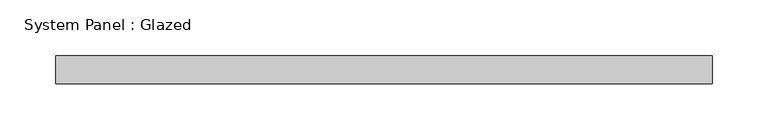
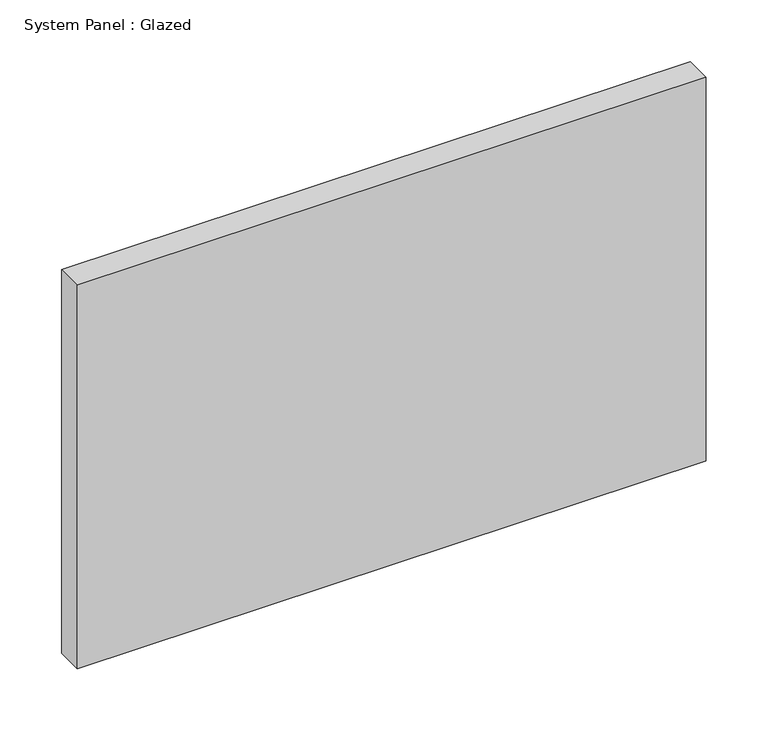
"""IFC4 building model written with IfcOpenShell, lengths in millimetres: plate geometry, System Panel : Glazed."""

from ifc_helpers import new_model, si_unit, origin, origin_with_axes, place, context, project, spatial, polyline, outline, extrude, source, transform, mapped, element, save


def system_panel_glazed_fa889304(model_context):
    return source(origin(), model_context, "Body", "SweptSolid", [
        extrude(outline(polyline([(295.275, 19.05), (-295.275, 19.05), (-295.275, 44.45), (295.275, 44.45), (295.275, 19.05)])), origin_with_axes(), (0.0, 0.0, 1.0), 381.0),
    ])


if __name__ == "__main__":
    model = new_model("IFC4")
    model_context = context("Model", 3, world=origin())
    ifc_project = project(units=[si_unit("LENGTHUNIT", "METRE", prefix="MILLI")], contexts=[model_context])
    site = spatial("IfcSite", under=ifc_project)
    building = spatial("IfcBuilding", under=site)
    placement = place(None, origin())
    system_panel_glazed_shape = system_panel_glazed_fa889304(model_context)
    element("IfcPlate", 1, ObjectType="System Panel : Glazed", at=placement, inside=building, context=model_context, shape_type="MappedRepresentation", body=[
        mapped(system_panel_glazed_shape, transform((0.0, 0.0, 0.0), x_axis=(1.0, 0.0, 0.0), y_axis=(0.0, 1.0, 0.0), z_axis=(0.0, 0.0, 1.0))),
    ])
    save(model, "model.ifc")

# Revit data of these elements
# Type "System Panel : Glazed"
#   Construction Type Id = "GSP4R"
#   Analytic Construction = "1/8 in Pilkington single glazing"
#   Visual Light Transmittance = 0.9
#   Solar Heat Gain Coefficient = 0.86
#   Heat Transfer Coefficient (U) = 1.18115 BTU/(h·ft²·°F)
#   Define Thermal Properties by = 1
# Element 1 (IfcPlate, "System Panel : Glazed")
#   Materials on its faces: "Glass"
# Materials
#   "Glass": class "Glass", colour RGB 0 128 192, transparency 0.75, Description = "Soda Lime Glass", Cost = 0
